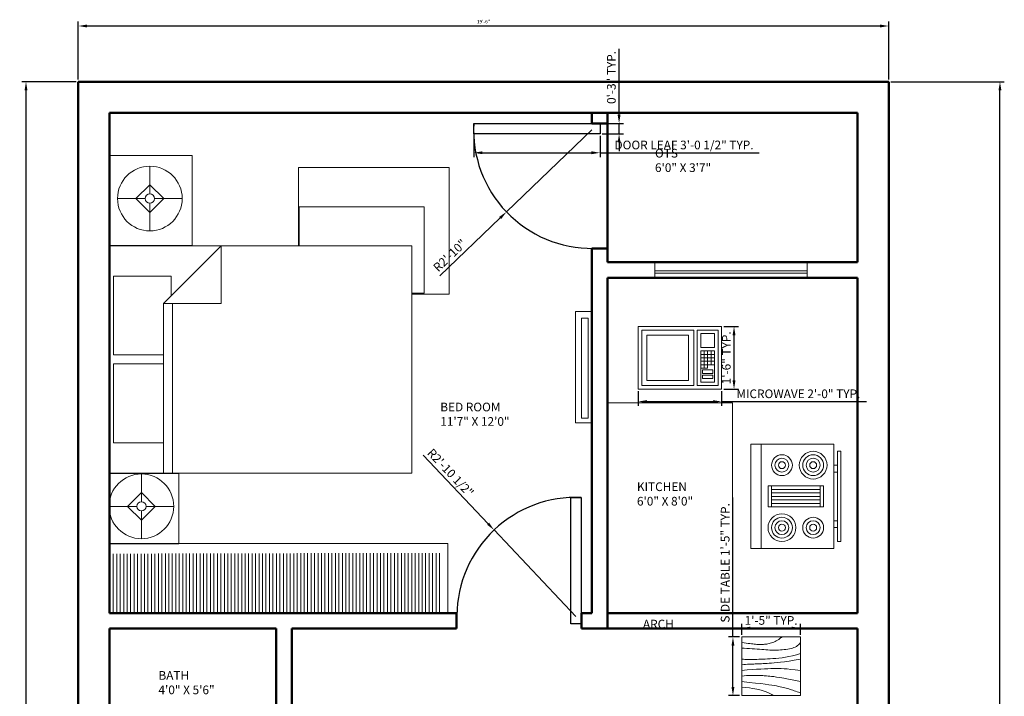
# Model space of a CAD drawing. Units: inches. Extents: x 210 to 950, y 0 to 561.
# Tile 5 of 5: x 635 to 919, y 366 to 561. Entities that reach past the tile are written whole.
import ezdxf

# ---------------------------------------------------------------- set-up
doc = ezdxf.new("R2010")
doc.units = ezdxf.units.IN
for name, color, linetype, lineweight in [('A-ANNO-DIMS', 2, 'Continuous', 18), ('A-ANNO-TEXT', 7, 'Continuous', 18), ('A-AREA-IDEN', 7, 'Continuous', 18), ('A-DOOR', 4, 'Continuous', 25), ('A-EQPM', 8, 'Continuous', 18), ('A-FLOR-CASE', 8, 'Continuous', 20), ('A-FURN', 8, 'Continuous', 18), ('A-FURN-PATT', 9, 'Continuous', 13), ('A-GLAZ', 4, 'Continuous', 20), ('A-WALL', 7, 'Continuous', 50)]:
    doc.layers.add(name, color=color, linetype=linetype, lineweight=lineweight)
doc.styles.get("Standard").update_dxf_attribs({"font": 'arial.ttf'})
doc.dimstyles.new('ISO-25', dxfattribs={"dimtxt": 2.5, "dimasz": 2.5, "dimexe": 1.25, "dimexo": 0.625, "dimtad": 1, "dimtxsty": 'Standard', "dimcen": 2.5, "dimadec": 0, "dimazin": 0, "dimtfac": 1, "dimtmove": 0, "dimatfit": 3, "dimfxl": 1, "dimarcsym": 0})

# ---------------------------------------------------------------- blocks, each defined once
blk = doc.blocks.new('Bed - Queen')
for p, q in [((0, -80.00003), (0, 0)), ((0, 0), (59.99999, 0)), ((59.99999, 0), (59.99999, -80.00003)), ((7.99999, -1.2), (28.79998, -1.2)), ((7.99999, -14.4), (7.99999, -1.2)), ((28.79998, -1.2), (28.79998, -14.4)), ((31.19999, -1.2), (51.99999, -1.2)), ((31.19999, -14.4), (31.19999, -1.2)), ((51.99999, -1.2), (51.99999, -16.4)), ((0, -14.4), (44.8, -14.4)), ((59.99999, -29.6), (44.8, -14.4)), ((44.8, -14.4), (44.8, -29.6)), ((44.8, -16.8), (0, -16.8)), ((51.99999, -16.4), (46.79936, -16.4)), ((44.8, -29.6), (59.99999, -29.6)), ((59.99999, -80.00003), (0, -80.00003))]:
    blk.add_line(p, q)
blk = doc.blocks.new('Lamp - Table')
for p, q in [((0, 7), (0, 1)), ((0, 3), (-3, 0)), ((3, 0), (0, 3)), ((-1, 0), (-7, 0)), ((-3, 0), (0, -3)), ((0, -3), (3, 0)), ((1, 0), (7, 0)), ((0, -1), (0, -7))]:
    blk.add_line(p, q)
for radius in [7, 1]:
    blk.add_circle((0, 0), radius)
blk = doc.blocks.new('Range-Oven - 30 in top')
for p, q in [((0, -3), (30, -3)), ((12, -6), (18, -6)), ((13, -20), (13, -6)), ((14, -6), (14, -20)), ((15, -20), (15, -6)), ((16, -6), (16, -20)), ((17, -20), (17, -6)), ((18, -20), (12, -20)), ((6, -24), (6, -25)), ((8, -25), (8, -24)), ((22, -25), (22, -24)), ((24, -24), (24, -25))]:
    blk.add_line(p, q)
for points in [[(0, -24), (0, 0), (30, 0), (30, -24)], [(12, -21), (12, -5), (18, -5), (18, -21)], [(2, -26), (2, -25), (28, -25), (28, -26)]]:
    blk.add_lwpolyline(points, close=True)
for centre, radius in [((6, -9), 4), ((6, -9), 3), ((6, -9), 2), ((6, -9), 1), ((24, -9), 3), ((24, -9), 2), ((24, -9), 1), ((24, -18), 4), ((6, -18), 3), ((6, -18), 2), ((6, -18), 1), ((24, -18), 3), ((24, -18), 2), ((24, -18), 1)]:
    blk.add_circle(centre, radius)
blk = doc.blocks.new('Microwave')
for p, q in [((18, 10), (22, 10)), ((22, 9), (18, 9)), ((19, 7), (19, 11)), ((20, 11), (20, 7)), ((21, 7), (21, 11)), ((18, 8), (22, 8)), ((22, 7), (18, 7)), ((20, 6), (18, 6)), ((19, 6), (19, 7)), ((20, 7), (20, 6))]:
    blk.add_line(p, q)
for points in [[(0, 0), (0, 18), (24, 18), (24, 0)], [(1, 1), (1, 17), (16, 17), (16, 1)], [(2.5, 2.5), (2.5, 15.5), (14.5, 15.5), (14.5, 2.5)], [(17, 1), (17, 17), (23, 17), (23, 1)], [(18, 12), (18, 16), (22, 16), (22, 12)], [(18, 2), (18, 11), (22, 11), (22, 2)], [(18.5, 4.5), (18.5, 5.5), (21.5, 5.5), (21.5, 4.5)], [(18.5, 3), (18.5, 4), (21.5, 4), (21.5, 3)]]:
    blk.add_lwpolyline(points, close=True)
blk = doc.blocks.new('Table - Square Woodgrain 42 x 42 in.')
blk.add_line((0, -42), (42, -42))
for points in [[(0, -4), (1.704, -4.2172), (3.2358, -4.4188), (4.615, -4.604), (5.8615, -4.7721), (6.9951, -4.9224), (8.0357, -5.0541), (9.0031, -5.1667), (9.9171, -5.2594), (10.7951, -5.3316), (11.6445, -5.3836), (12.4702, -5.4157), (13.277, -5.4283), (14.0698, -5.4217), (14.8535, -5.3964), (15.6331, -5.3526), (16.4133, -5.2908), (17.1986, -5.2103), (17.9913, -5.1062), (18.793, -4.9727), (19.6056, -4.8038), (20.4307, -4.5937), (21.2701, -4.3365), (22.1256, -4.0262), (22.9989, -3.6571), (23.888, -3.2272), (24.7756, -2.7516), (25.6408, -2.2491), (26.4624, -1.7387), (27.2195, -1.2395), (27.891, -0.7703), (28.456, -0.3501), (28.8934, 0.002)], [(0, -42), (0, 0), (42, 0), (42, -42)], [(0, -8), (1.8203, -8.1001), (3.6741, -8.2149), (5.5411, -8.3408), (7.4011, -8.4741), (9.2339, -8.6112), (11.0193, -8.7484), (12.7371, -8.8821), (14.3671, -9.0086), (15.8954, -9.1246), (17.3337, -9.2278), (18.6997, -9.3159), (20.0116, -9.387), (21.2871, -9.4389), (22.5442, -9.4696), (23.8008, -9.477), (25.0749, -9.459), (26.3791, -9.4137), (27.7049, -9.3403), (29.0383, -9.2382), (30.3655, -9.1068), (31.6728, -8.9455), (32.9461, -8.7535), (34.1717, -8.5304), (35.3358, -8.2756), (36.4268, -7.9863), (37.443, -7.6521), (38.3849, -7.2603), (39.253, -6.7986), (40.048, -6.2542), (40.7705, -5.6147), (41.421, -4.8674), (42, -4)], [(42, -12), (39.1784, -12.8621), (36.4519, -13.5654), (33.8246, -14.1294), (31.3004, -14.5731), (28.8832, -14.9161), (26.577, -15.1775), (24.3858, -15.3768), (22.3136, -15.5332), (20.3622, -15.6632), (18.5254, -15.7718), (16.7947, -15.8612), (15.1618, -15.9338), (13.6183, -15.9916), (12.1558, -16.0369), (10.7659, -16.0718), (9.4403, -16.0987), (8.1703, -16.1191), (6.9461, -16.1325), (5.7577, -16.1377), (4.595, -16.1335), (3.4479, -16.1188), (2.3064, -16.0924), (1.1604, -16.0532), (0, -16)], [(42, -16), (37.6529, -16.7365), (33.8802, -17.329), (30.6179, -17.7961), (27.8015, -18.1561), (25.3668, -18.4275), (23.2497, -18.6288), (21.3859, -18.7785), (19.7111, -18.8949), (18.1693, -18.9939), (16.7375, -19.0795), (15.401, -19.1534), (14.1449, -19.217), (12.9544, -19.2717), (11.8148, -19.3191), (10.7113, -19.3606), (9.6291, -19.3976), (8.5534, -19.4323), (7.47, -19.4689), (6.3643, -19.5122), (5.222, -19.5672), (4.0288, -19.6386), (2.7703, -19.7313), (1.4321, -19.8501), (0, -20)], [(0, -24), (3.9243, -23.6805), (7.4766, -23.4138), (10.6891, -23.1954), (13.5943, -23.0205), (16.2247, -22.8847), (18.6125, -22.7832), (20.7903, -22.7116), (22.7903, -22.6651), (24.6563, -22.642), (26.4764, -22.6507), (28.35, -22.7024), (30.3766, -22.8084), (32.6555, -22.98), (35.2861, -23.2283), (38.3678, -23.5645), (42, -24)], [(42, -32), (37.392, -31.017), (33.4585, -30.2231), (30.1291, -29.5949), (27.3334, -29.109), (25.0009, -28.742), (23.0612, -28.4707), (21.4439, -28.2716), (20.0786, -28.1215), (18.8998, -28.0002), (17.8609, -27.9014), (16.9206, -27.8219), (16.0371, -27.7588), (15.1691, -27.709), (14.2748, -27.6693), (13.3128, -27.6368), (12.2415, -27.6083), (11.0295, -27.5824), (9.6867, -27.5643), (8.233, -27.5608), (6.6884, -27.5787), (5.0728, -27.6248), (3.4062, -27.7058), (1.7086, -27.8286), (0, -28)], [(0, -32), (5.4026, -32.5358), (9.9494, -33.019), (13.7424, -33.4553), (16.8834, -33.8505), (19.4743, -34.2106), (21.6171, -34.5413), (23.4136, -34.8486), (24.9657, -35.1382), (26.3614, -35.4156), (27.6332, -35.6841), (28.7995, -35.9467), (29.8788, -36.2064), (30.8897, -36.4661), (31.8507, -36.7288), (32.7802, -36.9973), (33.6968, -37.2747), (34.6175, -37.5635), (35.5531, -37.8651), (36.5128, -38.1805), (37.506, -38.5108), (38.5421, -38.8568), (39.6302, -39.2197), (40.7797, -39.6004), (42, -40)], [(0, -36), (3.0098, -36.2857), (5.5354, -36.5643), (7.6368, -36.8359), (9.374, -37.1009), (10.807, -37.3597), (11.9957, -37.6126), (13.0002, -37.8599), (13.8804, -38.102), (14.6874, -38.3393), (15.4365, -38.5729), (16.1338, -38.8041), (16.7858, -39.0341), (17.3987, -39.264), (17.9787, -39.4952), (18.5322, -39.7288), (19.0655, -39.9662), (19.5832, -40.2081), (20.0842, -40.4544), (20.5657, -40.7046), (21.0249, -40.9581), (21.459, -41.2144), (21.8653, -41.4731), (22.2409, -41.7335), (22.5831, -41.9951)]]:
    blk.add_lwpolyline(points)
blk = doc.blocks.new('*D17')
at = {"layer": 'A-ANNO-DIMS', "color": 0, "lineweight": -2, "transparency": 16777216}
for p, q in [((651.28, 543.37), (635.61, 543.37)), ((636.86, 38.87), (636.86, 540.87)), ((651.28, 36.37), (635.61, 36.37))]:
    blk.add_line(p, q, dxfattribs=at)
at = {"layer": 'A-ANNO-DIMS', "color": 0, "transparency": 16777216}
for points in [[(636.44, 540.87), (637.27, 540.87), (636.86, 543.37)], [(636.44, 38.87), (637.27, 38.87), (636.86, 36.37)]]:
    blk.add_solid(points, dxfattribs=at)
at = {"layer": 'Defpoints', "color": 0, "transparency": 16777216}
for p in [(636.86, 543.37), (651.91, 543.37), (651.91, 36.37)]:
    blk.add_point(p, dxfattribs=at)
at = {"layer": 'A-ANNO-DIMS', "color": 0, "transparency": 16777216, "insert": (635.72, 289.87), "char_height": 1, "attachment_point": 5, "rotation": 90}
blk.add_mtext('42\'-3"', dxfattribs=at)
blk = doc.blocks.new('*D18')
at = {"layer": 'A-ANNO-DIMS', "color": 0, "lineweight": -2, "transparency": 16777216}
for p, q in [((651.91, 543.99), (651.91, 560.67)), ((654.41, 559.42), (882.91, 559.42)), ((885.41, 543.99), (885.41, 560.67))]:
    blk.add_line(p, q, dxfattribs=at)
at = {"layer": 'A-ANNO-DIMS', "color": 0, "transparency": 16777216}
for points in [[(654.41, 559.83), (654.41, 559), (651.91, 559.42)], [(882.91, 559.83), (882.91, 559), (885.41, 559.42)]]:
    blk.add_solid(points, dxfattribs=at)
at = {"layer": 'Defpoints', "color": 0, "transparency": 16777216}
for p in [(885.41, 559.42), (651.91, 543.37), (885.41, 543.37)]:
    blk.add_point(p, dxfattribs=at)
at = {"layer": 'A-ANNO-DIMS', "color": 0, "transparency": 16777216, "insert": (768.66, 560.55), "char_height": 1, "attachment_point": 5}
blk.add_mtext('19\'-6"', dxfattribs=at)
blk = doc.blocks.new('*D19')
at = {"layer": 'A-ANNO-DIMS', "color": 0, "lineweight": -2, "transparency": 16777216}
for p, q in [((886.03, 543.37), (918.72, 543.37)), ((917.47, 38.87), (917.47, 540.87)), ((886.03, 36.37), (918.72, 36.37))]:
    blk.add_line(p, q, dxfattribs=at)
at = {"layer": 'A-ANNO-DIMS', "color": 0, "transparency": 16777216}
for points in [[(917.05, 540.87), (917.89, 540.87), (917.47, 543.37)], [(917.05, 38.87), (917.89, 38.87), (917.47, 36.37)]]:
    blk.add_solid(points, dxfattribs=at)
at = {"layer": 'Defpoints', "color": 0, "transparency": 16777216}
for p in [(885.41, 543.37), (917.47, 543.37), (885.41, 36.37)]:
    blk.add_point(p, dxfattribs=at)
at = {"layer": 'A-ANNO-DIMS', "color": 0, "transparency": 16777216, "insert": (916.33, 289.87), "char_height": 1, "attachment_point": 5, "rotation": 90}
blk.add_mtext('42\'-3"', dxfattribs=at)
blk = doc.blocks.new('DOOR-LEAF-36IN')
blk.add_lwpolyline([(0, 0), (0, -2.99), (-36.41, -2.99), (-36.41, 0)], close=True)
blk = doc.blocks.new('*D22')
at = {"layer": 'A-ANNO-DIMS', "color": 0, "lineweight": -2, "transparency": 16777216}
for p, q in [((765.86, 527.75), (765.86, 521.66)), ((802.27, 527.75), (802.27, 521.66)), ((768.36, 522.91), (799.77, 522.91)), ((802.27, 522.91), (848.11, 522.91))]:
    blk.add_line(p, q, dxfattribs=at)
at = {"layer": 'A-ANNO-DIMS', "color": 0, "transparency": 16777216}
for points in [[(768.36, 523.33), (768.36, 522.5), (765.86, 522.91)], [(799.77, 523.33), (799.77, 522.5), (802.27, 522.91)]]:
    blk.add_solid(points, dxfattribs=at)
at = {"layer": 'Defpoints', "color": 0, "transparency": 16777216}
for p in [(765.86, 528.37), (802.27, 528.37), (802.27, 522.91)]:
    blk.add_point(p, dxfattribs=at)
at = {"layer": 'A-ANNO-DIMS', "color": 0, "transparency": 16777216, "insert": (826.44, 524.83), "char_height": 2.5, "attachment_point": 5}
blk.add_mtext('DOOR LEAF 3\'-0 1/2" TYP.', dxfattribs=at)
blk = doc.blocks.new('*D23')
at = {"layer": 'A-ANNO-DIMS', "color": 0, "lineweight": -2, "transparency": 16777216}
for p, q in [((807.73, 533.86), (807.73, 552.85)), ((802.9, 531.36), (808.98, 531.36)), ((807.73, 528.37), (807.73, 531.36)), ((802.9, 528.37), (808.98, 528.37)), ((807.73, 525.87), (807.73, 523.37))]:
    blk.add_line(p, q, dxfattribs=at)
at = {"layer": 'A-ANNO-DIMS', "color": 0, "transparency": 16777216}
for points in [[(807.32, 533.86), (808.15, 533.86), (807.73, 531.36)], [(807.32, 525.87), (808.15, 525.87), (807.73, 528.37)]]:
    blk.add_solid(points, dxfattribs=at)
at = {"layer": 'Defpoints', "color": 0, "transparency": 16777216}
for p in [(802.27, 531.36), (807.73, 531.36), (802.27, 528.37)]:
    blk.add_point(p, dxfattribs=at)
at = {"layer": 'A-ANNO-DIMS', "color": 0, "transparency": 16777216, "insert": (805.83, 544.6), "char_height": 2.5, "attachment_point": 5, "rotation": 90}
blk.add_mtext('0\'-3" TYP.', dxfattribs=at)
blk = doc.blocks.new('*D32')
at = {"layer": 'A-ANNO-DIMS', "color": 0, "lineweight": -2, "transparency": 16777216}
for p, q in [((840.54, 383.49), (840.54, 423.62)), ((842.45, 383.49), (839.29, 383.49)), ((840.54, 369.1), (840.54, 380.99)), ((842.45, 366.6), (839.29, 366.6))]:
    blk.add_line(p, q, dxfattribs=at)
at = {"layer": 'A-ANNO-DIMS', "color": 0, "transparency": 16777216}
for points in [[(840.12, 380.99), (840.95, 380.99), (840.54, 383.49)], [(840.12, 369.1), (840.95, 369.1), (840.54, 366.6)]]:
    blk.add_solid(points, dxfattribs=at)
at = {"layer": 'Defpoints', "color": 0, "transparency": 16777216}
for p in [(840.54, 383.49), (843.07, 383.49), (843.07, 366.6)]:
    blk.add_point(p, dxfattribs=at)
at = {"layer": 'A-ANNO-DIMS', "color": 0, "transparency": 16777216, "insert": (838.62, 404.81), "char_height": 2.5, "attachment_point": 5, "rotation": 90}
blk.add_mtext('SIDE TABLE 1\'-5" TYP.', dxfattribs=at)
blk = doc.blocks.new('*D33')
at = {"layer": 'A-ANNO-DIMS', "color": 0, "lineweight": -2, "transparency": 16777216}
for p, q in [((843.07, 384.11), (843.07, 387.27)), ((845.57, 386.02), (857.46, 386.02)), ((859.96, 384.11), (859.96, 387.27))]:
    blk.add_line(p, q, dxfattribs=at)
at = {"layer": 'A-ANNO-DIMS', "color": 0, "transparency": 16777216}
for points in [[(845.57, 386.44), (845.57, 385.61), (843.07, 386.02)], [(857.46, 386.44), (857.46, 385.61), (859.96, 386.02)]]:
    blk.add_solid(points, dxfattribs=at)
at = {"layer": 'Defpoints', "color": 0, "transparency": 16777216}
for p in [(859.96, 386.02), (843.07, 383.49), (859.96, 383.49)]:
    blk.add_point(p, dxfattribs=at)
at = {"layer": 'A-ANNO-DIMS', "color": 0, "transparency": 16777216, "insert": (851.52, 387.92), "char_height": 2.5, "attachment_point": 5}
blk.add_mtext('1\'-5" TYP.', dxfattribs=at)
blk = doc.blocks.new('*D38')
at = {"layer": 'A-ANNO-DIMS', "color": 0, "lineweight": -2, "transparency": 16777216}
for p, q in [((813.25, 454.24), (813.25, 450.01)), ((837.25, 454.24), (837.25, 450.01)), ((815.75, 451.26), (834.75, 451.26)), ((837.25, 451.26), (879.02, 451.26))]:
    blk.add_line(p, q, dxfattribs=at)
at = {"layer": 'A-ANNO-DIMS', "color": 0, "transparency": 16777216}
for points in [[(815.75, 451.68), (815.75, 450.85), (813.25, 451.26)], [(834.75, 451.68), (834.75, 450.85), (837.25, 451.26)]]:
    blk.add_solid(points, dxfattribs=at)
at = {"layer": 'Defpoints', "color": 0, "transparency": 16777216}
for p in [(813.25, 454.86), (837.25, 454.86), (837.25, 451.26)]:
    blk.add_point(p, dxfattribs=at)
at = {"layer": 'A-ANNO-DIMS', "color": 0, "transparency": 16777216, "insert": (859.38, 453.18), "char_height": 2.5, "attachment_point": 5}
blk.add_mtext('MICROWAVE 2\'-0" TYP.', dxfattribs=at)
blk = doc.blocks.new('*D39')
at = {"layer": 'A-ANNO-DIMS', "color": 0, "lineweight": -2, "transparency": 16777216}
for p, q in [((837.87, 472.86), (842.1, 472.86)), ((840.85, 457.36), (840.85, 470.36)), ((837.87, 454.86), (842.1, 454.86))]:
    blk.add_line(p, q, dxfattribs=at)
at = {"layer": 'A-ANNO-DIMS', "color": 0, "transparency": 16777216}
for points in [[(840.43, 470.36), (841.27, 470.36), (840.85, 472.86)], [(840.43, 457.36), (841.27, 457.36), (840.85, 454.86)]]:
    blk.add_solid(points, dxfattribs=at)
at = {"layer": 'Defpoints', "color": 0, "transparency": 16777216}
for p in [(837.25, 472.86), (840.85, 472.86), (837.25, 454.86)]:
    blk.add_point(p, dxfattribs=at)
at = {"layer": 'A-ANNO-DIMS', "color": 0, "transparency": 16777216, "insert": (838.95, 463.86), "char_height": 2.5, "attachment_point": 5, "rotation": 90}
blk.add_mtext('1\'-6" TYP.', dxfattribs=at)
blk = doc.blocks.new('*D62')
at = {"layer": 'A-ANNO-DIMS', "color": 0, "lineweight": -2, "transparency": 16777216}
for p, q in [((751.33, 435.8), (769.98, 416.1)), ((795.31, 389.34), (771.7, 414.28))]:
    blk.add_line(p, q, dxfattribs=at)
at = {"layer": 'A-ANNO-DIMS', "color": 0, "transparency": 16777216}
blk.add_solid([(770.28, 416.39), (769.68, 415.81), (771.7, 414.28)], dxfattribs=at)
at = {"layer": 'Defpoints', "color": 0, "transparency": 16777216}
for p in [(771.7, 414.28), (795.31, 389.34)]:
    blk.add_point(p, dxfattribs=at)
at = {"layer": 'A-ANNO-DIMS', "color": 0, "transparency": 16777216, "insert": (758.93, 430.56), "char_height": 2.5, "attachment_point": 5, "rotation": 313.4284}
blk.add_mtext('R2\'-10 1/2"', dxfattribs=at)
blk = doc.blocks.new('*D64')
at = {"layer": 'A-ANNO-DIMS', "color": 0, "lineweight": -2, "transparency": 16777216}
for p, q in [((799.91, 529.47), (775.28, 505.88)), ((756.09, 487.51), (773.48, 504.16))]:
    blk.add_line(p, q, dxfattribs=at)
at = {"layer": 'A-ANNO-DIMS', "color": 0, "transparency": 16777216}
blk.add_solid([(773.19, 504.46), (773.76, 503.85), (775.28, 505.88)], dxfattribs=at)
at = {"layer": 'Defpoints', "color": 0, "transparency": 16777216}
for p in [(799.91, 529.47), (775.28, 505.88)]:
    blk.add_point(p, dxfattribs=at)
at = {"layer": 'A-ANNO-DIMS', "color": 0, "transparency": 16777216, "insert": (759.19, 493.11), "char_height": 2.5, "attachment_point": 5, "rotation": 43.7588}
blk.add_mtext('R2\'-10"', dxfattribs=at)

msp = doc.modelspace()

# ---------------------------------------------------------------- hatches: boundary and pattern name
at = {"layer": 'A-FURN-PATT'}
h = msp.add_hatch(dxfattribs=at)
h.set_pattern_fill('ANSI31', color=256, scale=0.3149606, angle=45, style=0)
h.paths.add_polyline_path([(756.43, 390.56), (756.43, 407.6), (731.43, 407.6), (661.1, 407.43), (661.1, 390.39), (679.21, 390.3), (704.21, 390.3)])

# ---------------------------------------------------------------- linework, layer by layer
at = {"layer": 'A-DOOR'}
for centre, radius, start, end in [((799.91, 529.47), 34.1, 176.8429, 270.6748), ((795.31, 389.34), 34.34, 87.4624, 179.3939)]:
    msp.add_arc(centre, radius, start, end, dxfattribs=at)
at = {"layer": 'A-FLOR-CASE'}
for p in [(804.41, 450.87), (840.41, 390.37)]:
    msp.add_line(p, (840.41, 450.87), dxfattribs=at)
msp.add_lwpolyline([(660.85, 390.44), (758.39, 390.44), (758.39, 410.39), (660.85, 410.39)], close=True, dxfattribs=at)
at = {"layer": 'A-FURN'}
for points in [[(660.99, 522.1), (684.71, 522.1), (684.71, 496.16), (660.99, 496.16)], [(799.74, 477.24), (795.14, 477.24), (795.14, 445.15), (799.74, 445.15)], [(798.81, 475.31), (796.86, 475.31), (796.86, 446.48), (798.81, 446.48)], [(660.9, 430.59), (680.92, 430.59), (680.92, 410.29), (660.9, 410.29)]]:
    msp.add_lwpolyline(points, close=True, dxfattribs=at)
for points in [[(715.35, 496.12), (715.35, 518.65), (758.82, 518.65), (758.82, 482.23), (748.02, 482.23)], [(715.57, 496.12), (715.57, 507.39), (751.58, 507.39), (751.58, 482.47), (748.02, 482.47)]]:
    msp.add_lwpolyline(points, dxfattribs=at)
at = {"layer": 'A-GLAZ'}
for p, q in [((818, 486.87), (818, 491.27)), ((818, 491.27), (861.9, 491.27)), ((861.9, 491.27), (861.9, 486.87)), ((818, 488.87), (861.9, 488.87)), ((861.9, 488.27), (818, 488.27))]:
    msp.add_line(p, q, dxfattribs=at)
at = {"layer": 'A-WALL'}
for p, q in [((651.91, 36.37), (651.91, 543.37)), ((651.91, 543.37), (885.41, 543.37)), ((885.41, 36.37), (885.41, 543.37)), ((660.91, 534.37), (876.41, 534.37)), ((660.91, 390.37), (660.91, 534.37)), ((799.91, 531.37), (799.91, 534.37)), ((804.41, 531.37), (804.41, 534.37)), ((876.41, 491.37), (876.41, 534.37)), ((876.41, 491.37), (876.41, 534.37)), ((799.91, 531.37), (804.41, 531.37)), ((804.41, 491.37), (804.41, 531.37)), ((799.91, 390.37), (799.91, 495.37)), ((799.91, 495.37), (804.41, 495.37)), ((804.41, 491.37), (876.41, 491.37)), ((804.41, 385.87), (804.41, 486.87)), ((804.41, 486.87), (876.41, 486.87)), ((876.41, 390.37), (876.41, 486.87)), ((876.41, 390.37), (876.41, 486.87)), ((660.91, 390.37), (760.91, 390.37)), ((760.91, 385.87), (760.91, 390.37)), ((796.91, 385.87), (796.91, 390.37)), ((796.91, 390.37), (799.91, 390.37)), ((804.41, 390.37), (876.41, 390.37)), ((660.91, 385.87), (708.91, 385.87)), ((660.91, 315.37), (660.91, 385.87)), ((708.91, 319.87), (708.91, 385.87)), ((713.41, 315.37), (713.41, 385.87)), ((713.41, 268.87), (713.41, 385.87)), ((713.41, 220.87), (713.41, 385.87)), ((713.41, 385.87), (760.91, 385.87)), ((796.91, 385.87), (876.41, 385.87)), ((876.41, 81.37), (876.41, 385.87))]:
    msp.add_line(p, q, dxfattribs=at)

# ---------------------------------------------------------------- block references
at = {"layer": 'A-DOOR'}
msp.add_blockref('DOOR-LEAF-36IN', (802.27, 531.36), dxfattribs=at)
at = {"layer": 'A-DOOR', "rotation": 270}
msp.add_blockref('DOOR-LEAF-36IN', (796.83, 387.24), dxfattribs=at)
at = {"layer": 'A-EQPM'}
msp.add_blockref('Microwave', (813.25, 454.86), dxfattribs=at)
at = {"layer": 'A-EQPM', "rotation": 90}
msp.add_blockref('Range-Oven - 30 in top', (845.65, 408.95), dxfattribs=at)
at = {"layer": 'A-FURN'}
for name, p, xscale, yscale, zscale in [('Lamp - Table', (672.54, 509.73), 1.330786106251803, 1.330786106251803, 1.330786106251803), ('Lamp - Table', (670.11, 421.09), 1.330786106251803, 1.330786106251803, 1.330786106251803), ('Table - Square Woodgrain 42 x 42 in.', (843.07, 383.49), 0.4021241876100556, 0.4021241876100556, 0.4021241876100556)]:
    msp.add_blockref(name, p, dxfattribs=dict(at, xscale=xscale, yscale=yscale, zscale=zscale))
at = {"layer": 'A-FURN', "xscale": 1.090825566177695, "yscale": 1.090825566177695, "zscale": 1.090825566177695, "rotation": 90}
msp.add_blockref('Bed - Queen', (660.75, 430.67), dxfattribs=at)

# ---------------------------------------------------------------- texts
at = {"layer": 'A-ANNO-TEXT', "insert": (814.6, 388.43), "char_height": 2.5, "attachment_point": 1}
msp.add_mtext_dynamic_manual_height_columns('ARCH', width=3.9623, gutter_width=12.5, heights=[0], dxfattribs=at)
at = {"layer": 'A-AREA-IDEN', "char_height": 2.5, "attachment_point": 1}
for s, width, insert in [('OTS\\P6\'0" X 3\'7"', 45.646, (818.07, 524.04)), ('BED ROOM\\P11\'7" X 12\'0"', 30.2568, (756.21, 450.95)), ('KITCHEN\\P6\'0" X 8\'0"', 16.3552, (812.88, 427.99)), ('BATH\\P\\pxt10;4\'0" X 5\'6" ', 26.7357, (675.02, 373.65))]:
    msp.add_mtext_dynamic_manual_height_columns(s, width=width, gutter_width=12.5, heights=[0], dxfattribs=dict(at, insert=insert))

# ---------------------------------------------------------------- dimensions: what is measured, and where the dimension line sits
at = {"layer": 'A-ANNO-DIMS'}
dim = msp.add_linear_dim(base=(885.40828592, 559.41590781), p1=(651.90828592, 543.36597025), p2=(885.40828592, 543.36597025), dimstyle='ISO-25', override={"dimtxt": 1, "dimdec": 0, "dimlunit": 3, "dimclrd": 0, "dimclre": 0, "dimclrt": 0, "dimtdec": 0}, dxfattribs=at)
dim.commit()
dim.dimension.update_dxf_attribs({"geometry": '*D18', "text_midpoint": (768.65828592, 560.5514808)})
for base, p1, p2, text, picture, middle in [((807.73, 531.36), (802.27, 528.37), (802.27, 531.36), '<> TYP.', '*D23', (805.83, 544.6)), ((840.85, 472.86), (837.25, 454.86), (837.25, 472.86), '<> TYP.', '*D39', (838.95, 463.86)), ((840.54, 383.49), (843.07, 366.6), (843.07, 383.49), 'SIDE TABLE <> TYP.', '*D32', (838.62, 404.81))]:
    dim = msp.add_linear_dim(base=base, p1=p1, p2=p2, angle=90, text=text, dimstyle='ISO-25', override={"dimdec": 1, "dimlfac": 1, "dimrnd": 0, "dimzin": 1, "dimdsep": 46, "dimlunit": 4, "dimfrac": 2}, dxfattribs=at)
    dim.commit()
    dim.dimension.update_dxf_attribs({"geometry": picture, "text_midpoint": middle})
for base, p1, p2, picture, middle in [((636.86, 543.37), (651.91, 36.37), (651.91, 543.37), '*D17', (635.72, 289.87)), ((917.47, 543.37), (885.41, 36.37), (885.41, 543.37), '*D19', (916.33, 289.87))]:
    dim = msp.add_linear_dim(base=base, p1=p1, p2=p2, angle=90, dimstyle='ISO-25', override={"dimtxt": 1, "dimdec": 0, "dimlunit": 3, "dimclrd": 0, "dimclre": 0, "dimclrt": 0, "dimtdec": 0}, dxfattribs=at)
    dim.commit()
    dim.dimension.update_dxf_attribs({"geometry": picture, "text_midpoint": middle})
for base, p1, p2, text, picture, middle in [((802.27, 522.91), (765.86, 528.37), (802.27, 528.37), 'DOOR LEAF <> TYP.', '*D22', (826.44, 524.83)), ((837.25, 451.26), (813.25, 454.86), (837.25, 454.86), 'MICROWAVE <> TYP.', '*D38', (859.38, 453.18)), ((859.96, 386.02), (843.07, 383.49), (859.96, 383.49), '<> TYP.', '*D33', (851.52, 387.92))]:
    dim = msp.add_linear_dim(base=base, p1=p1, p2=p2, text=text, dimstyle='ISO-25', override={"dimdec": 1, "dimlfac": 1, "dimrnd": 0, "dimzin": 1, "dimdsep": 46, "dimlunit": 4, "dimfrac": 2}, dxfattribs=at)
    dim.commit()
    dim.dimension.update_dxf_attribs({"geometry": picture, "text_midpoint": middle})
for center, mpoint, picture, middle in [((799.91, 529.47), (775.28, 505.88), '*D64', (760.51, 491.74)), ((795.31, 389.34), (771.7, 414.28), '*D62', (757.53, 429.25))]:
    dim = msp.add_radius_dim(center=center, mpoint=mpoint, dimstyle='ISO-25', override={"dimdec": 1, "dimlfac": 1, "dimrnd": 0, "dimzin": 1, "dimdsep": 46, "dimlunit": 4, "dimfrac": 2}, dxfattribs=at)
    dim.commit()
    dim.dimension.update_dxf_attribs({"geometry": picture, "text_midpoint": middle, "dimtype": 164})

doc.saveas('drawing.dxf')
